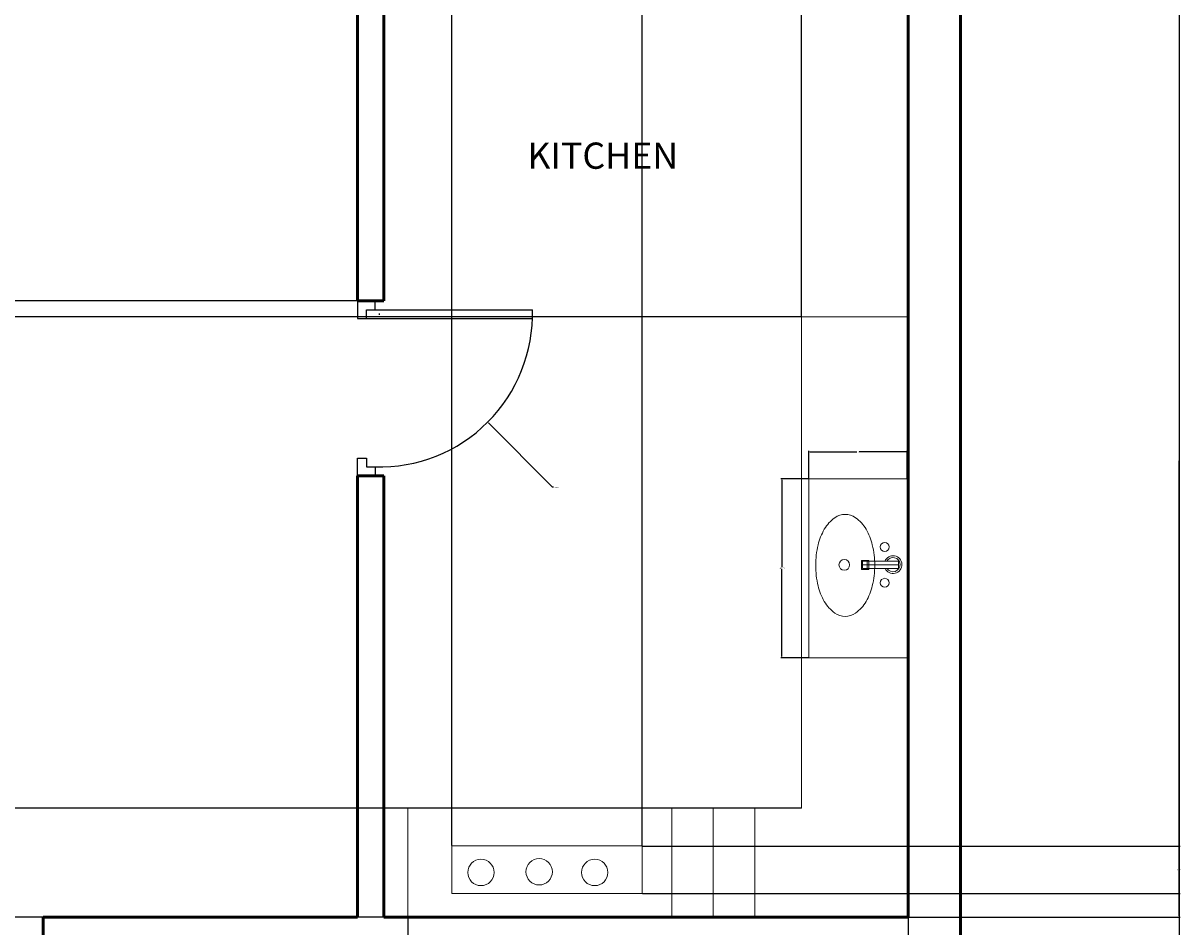
# Model space of a CAD drawing. Units: inches. Extents: x 1865 to 2541, y 1997 to 2759.
# Tile 10 of 11: x 2342 to 2541, y 2405 to 2560. Entities that reach past the tile are written whole.
import ezdxf

# ---------------------------------------------------------------- set-up
doc = ezdxf.new("R2010")
doc.units = ezdxf.units.IN
for name, color, linetype, lineweight in [('A-ANNO-DIMS', 2, 'Continuous', 18), ('A-AREA-IDEN', 4, 'Continuous', 18), ('A-EQPM', 8, 'Continuous', 18), ('A-FLOR-CASE', 8, 'Continuous', 20), ('A-FLOR-FIXT', 9, 'Continuous', 18), ('A-WALL', 7, 'Continuous', 50), ('DOOR', 1, 'Continuous', 25)]:
    doc.layers.add(name, color=color, linetype=linetype, lineweight=lineweight)
doc.styles.get("Standard").update_dxf_attribs({"font": 'arial.ttf'})
doc.dimstyles.get("Standard").update_dxf_attribs({"dimtxt": 0.18, "dimasz": 0.18, "dimexe": 0.18, "dimexo": 0.0625, "dimgap": 0.09, "dimtad": 0, "dimtih": 1, "dimtoh": 1, "dimdec": 4, "dimzin": 0, "dimdsep": 46, "dimtxsty": 'Standard', "dimcen": 0.09, "dimadec": 0, "dimazin": 0, "dimtfac": 1, "dimtdec": 4, "dimtofl": 0, "dimtmove": 0, "dimatfit": 3, "dimfxl": 1, "dimtolj": 1, "dimtzin": 0, "dimarcsym": 0})

# ---------------------------------------------------------------- blocks, each defined once
blk = doc.blocks.new('A$C50A015BB')
for p, q in [((0, 0.55), (1, 0.55)), ((0, 0.55), (0, 0)), ((1, 0.55), (1, 0)), ((0.4985, 0.5), (0.5385, 0.5)), ((0.4985, 0.5), (0.4985, 0.3)), ((0.5185, 0.5), (0.5185, 0.3)), ((0.5385, 0.5), (0.5385, 0.3)), ((0.4935, 0.335), (0.4935, 0.295)), ((0.4935, 0.335), (0.5435, 0.335)), ((0.4985, 0.325), (0.5385, 0.325)), ((0.5435, 0.335), (0.5435, 0.295)), ((0.4935, 0.295), (0.5435, 0.295)), ((0.4985, 0.3), (0.5385, 0.3)), ((0, 0), (1, 0)), ((0, 0), (1, 0))]:
    blk.add_line(p, q)
for centre, radius in [((0.4185, 0.424), 0.025), ((0.6185, 0.424), 0.025), ((0.5185, 0.1981), 0.0298)]:
    blk.add_circle(centre, radius)
for centre, radius, start, end in [((0.5201, 0.4703), 0.0497, 291.74253, 244.23308), ((0.5201, 0.4703), 0.0397, 297.63203, 237.02558), ((0.4772, 0.0383), 0.3252, 103.48533, 120.06859), ((0.5157, -0.1225), 0.4906, 90, 103.48533), ((0.5157, -0.1225), 0.4906, 76.51467, 90), ((0.5543, 0.0383), 0.3252, 59.93141, 76.51467), ((0.3299, 0.2031), 0.0991, 144.41781, 180), ((0.4185, 0.1397), 0.2081, 120.06859, 144.41781), ((0.613, 0.1397), 0.2081, 35.58219, 59.93141), ((0.7016, 0.2031), 0.0991, 0, 35.58219), ((0.3299, 0.2031), 0.0991, 180, 215.58219), ((0.7016, 0.2031), 0.0991, 324.41781, 0), ((0.4185, 0.2665), 0.2081, 215.58219, 239.93141), ((0.613, 0.2665), 0.2081, 300.06859, 324.41781), ((0.4772, 0.3679), 0.3252, 239.93141, 256.51467), ((0.5543, 0.3679), 0.3252, 283.48533, 300.06859), ((0.5157, 0.5288), 0.4906, 256.51467, 270), ((0.5157, 0.5288), 0.4906, 270, 283.48533)]:
    blk.add_arc(centre, radius, start, end)
blk = doc.blocks.new('DOOR-SWING-30IN')
for p, q in [((3, 30), (0, 30)), ((0, 30), (0, 27)), ((3, 28.5), (3, 30)), ((1.5, 27), (1.5, 28.5)), ((1.5, 28.5), (3, 28.5)), ((1.5, 28.5), (30, 28.5)), ((0, 27), (1.5, 27)), ((0, 27), (30, 27)), ((0, 0), (0, 3)), ((0, 3), (1.5, 3)), ((1.5, 3), (1.5, 1.5)), ((1.5, 1.5), (3, 1.5)), ((3, 1.5), (3, 0)), ((3, 0), (0, 0))]:
    blk.add_line(p, q)
blk.add_arc((3.75, 27.75), 26.26, 268.3634, 1.6366)
blk = doc.blocks.new('*D28')
at = {"layer": 'A-ANNO-DIMS', "color": 0, "lineweight": -2, "transparency": 16777216}
for p, q in [((2477.13, 2482.2), (2472.4, 2482.2)), ((2472.58, 2482.02), (2472.58, 2467.02)), ((2472.58, 2451.65), (2472.58, 2466.65)), ((2477.13, 2451.47), (2472.4, 2451.47))]:
    blk.add_line(p, q, dxfattribs=at)
at = {"layer": 'A-ANNO-DIMS', "color": 0, "transparency": 16777216}
for points in [[(2472.55, 2482.02), (2472.61, 2482.02), (2472.58, 2482.2)], [(2472.55, 2451.65), (2472.61, 2451.65), (2472.58, 2451.47)]]:
    blk.add_solid(points, dxfattribs=at)
at = {"layer": 'Defpoints', "color": 0, "transparency": 16777216}
for p in [(2472.58, 2482.2), (2477.19, 2482.2), (2477.19, 2451.47)]:
    blk.add_point(p, dxfattribs=at)
at = {"layer": 'A-ANNO-DIMS', "color": 0, "transparency": 16777216, "insert": (2472.58, 2466.83), "char_height": 0.18, "attachment_point": 5}
blk.add_mtext('\\A1;SINK 31', dxfattribs=at)
blk = doc.blocks.new('*D29')
at = {"layer": 'A-ANNO-DIMS', "color": 0, "lineweight": -2, "transparency": 16777216}
for p, q in [((2477.19, 2482.26), (2477.19, 2486.99)), ((2477.37, 2486.81), (2485.44, 2486.81)), ((2493.92, 2486.81), (2485.86, 2486.81)), ((2494.1, 2482.26), (2494.1, 2486.99))]:
    blk.add_line(p, q, dxfattribs=at)
at = {"layer": 'A-ANNO-DIMS', "color": 0, "transparency": 16777216}
for points in [[(2477.37, 2486.84), (2477.37, 2486.78), (2477.19, 2486.81)], [(2493.92, 2486.84), (2493.92, 2486.78), (2494.1, 2486.81)]]:
    blk.add_solid(points, dxfattribs=at)
at = {"layer": 'Defpoints', "color": 0, "transparency": 16777216}
for p in [(2494.1, 2486.81), (2477.19, 2482.2), (2494.1, 2482.2)]:
    blk.add_point(p, dxfattribs=at)
at = {"layer": 'A-ANNO-DIMS', "color": 0, "transparency": 16777216, "insert": (2485.65, 2486.81), "char_height": 0.18, "attachment_point": 5}
blk.add_mtext('\\A1;17', dxfattribs=at)
blk = doc.blocks.new('*D41')
at = {"layer": 'A-ANNO-DIMS', "color": 0, "lineweight": -2, "transparency": 16777216}
for p, q in [((2503.31, 2721.45), (2540.92, 2721.45)), ((2540.74, 2721.27), (2540.74, 2378.49)), ((2540.74, 2035.35), (2540.74, 2378.13)), ((2136.19, 2035.17), (2540.92, 2035.17))]:
    blk.add_line(p, q, dxfattribs=at)
at = {"layer": 'A-ANNO-DIMS', "color": 0, "transparency": 16777216}
for points in [[(2540.71, 2721.27), (2540.77, 2721.27), (2540.74, 2721.45)], [(2540.71, 2035.35), (2540.77, 2035.35), (2540.74, 2035.17)]]:
    blk.add_solid(points, dxfattribs=at)
at = {"layer": 'Defpoints', "color": 0, "transparency": 16777216}
for p in [(2503.24, 2721.45), (2136.13, 2035.17), (2540.74, 2035.17)]:
    blk.add_point(p, dxfattribs=at)
at = {"layer": 'A-ANNO-DIMS', "color": 0, "transparency": 16777216, "insert": (2540.74, 2378.31), "char_height": 0.18, "attachment_point": 5}
blk.add_mtext('\\A1;686.3', dxfattribs=at)
blk = doc.blocks.new('*D62')
at = {"layer": 'A-ANNO-DIMS', "color": 0, "lineweight": -2, "transparency": 16777216}
for p, q in [((2494.31, 2563.95), (2540.92, 2563.95)), ((2540.74, 2563.77), (2540.74, 2485.63)), ((2540.74, 2407.13), (2540.74, 2485.27)), ((2494.31, 2406.95), (2540.92, 2406.95))]:
    blk.add_line(p, q, dxfattribs=at)
at = {"layer": 'A-ANNO-DIMS', "color": 0, "transparency": 16777216}
for points in [[(2540.71, 2563.77), (2540.77, 2563.77), (2540.74, 2563.95)], [(2540.71, 2407.13), (2540.77, 2407.13), (2540.74, 2406.95)]]:
    blk.add_solid(points, dxfattribs=at)
at = {"layer": 'Defpoints', "color": 0, "transparency": 16777216}
for p in [(2494.24, 2563.95), (2540.74, 2563.95), (2494.24, 2406.95)]:
    blk.add_point(p, dxfattribs=at)
at = {"layer": 'A-ANNO-DIMS', "color": 0, "transparency": 16777216, "insert": (2540.74, 2485.45), "char_height": 0.18, "attachment_point": 5}
blk.add_mtext('\\A1;157', dxfattribs=at)
blk = doc.blocks.new('*D63')
at = {"layer": 'A-ANNO-DIMS', "color": 0, "lineweight": -2, "transparency": 16777216}
for p, q in [((2404.18, 2563.95), (1865.56, 2563.95)), ((1865.74, 2563.77), (1865.74, 2538.51)), ((1865.74, 2512.9), (1865.74, 2538.15)), ((2404.18, 2512.72), (1865.56, 2512.72))]:
    blk.add_line(p, q, dxfattribs=at)
at = {"layer": 'A-ANNO-DIMS', "color": 0, "transparency": 16777216}
for points in [[(1865.71, 2563.77), (1865.77, 2563.77), (1865.74, 2563.95)], [(1865.71, 2512.9), (1865.77, 2512.9), (1865.74, 2512.72)]]:
    blk.add_solid(points, dxfattribs=at)
at = {"layer": 'Defpoints', "color": 0, "transparency": 16777216}
for p in [(2404.24, 2563.95), (1865.74, 2512.72), (2404.24, 2512.72)]:
    blk.add_point(p, dxfattribs=at)
at = {"layer": 'A-ANNO-DIMS', "color": 0, "transparency": 16777216, "insert": (1865.74, 2538.33), "char_height": 0.18, "attachment_point": 5}
blk.add_mtext('\\A1;51.23', dxfattribs=at)
blk = doc.blocks.new('*D64')
at = {"layer": 'A-ANNO-DIMS', "color": 0, "lineweight": -2, "transparency": 16777216}
for p, q in [((2408.38, 2406.89), (2408.38, 1997.49)), ((2494.24, 2406.89), (2494.24, 1997.49)), ((2408.56, 1997.67), (2450.92, 1997.67)), ((2494.06, 1997.67), (2451.7, 1997.67))]:
    blk.add_line(p, q, dxfattribs=at)
at = {"layer": 'A-ANNO-DIMS', "color": 0, "transparency": 16777216}
for points in [[(2408.56, 1997.7), (2408.56, 1997.64), (2408.38, 1997.67)], [(2494.06, 1997.7), (2494.06, 1997.64), (2494.24, 1997.67)]]:
    blk.add_solid(points, dxfattribs=at)
at = {"layer": 'Defpoints', "color": 0, "transparency": 16777216}
for p in [(2408.38, 2406.95), (2494.24, 2406.95), (2494.24, 1997.67)]:
    blk.add_point(p, dxfattribs=at)
at = {"layer": 'A-ANNO-DIMS', "color": 0, "transparency": 16777216, "insert": (2451.31, 1997.67), "char_height": 0.18, "attachment_point": 5}
blk.add_mtext('\\A1;85.87', dxfattribs=at)
blk = doc.blocks.new('*D65')
at = {"layer": 'A-ANNO-DIMS', "color": 0, "lineweight": -2, "transparency": 16777216}
for p, q in [((2475.95, 2510.05), (2475.95, 2759.13)), ((2476.13, 2758.95), (2484.71, 2758.95)), ((2494.06, 2758.95), (2485.48, 2758.95)), ((2494.24, 2510.05), (2494.24, 2759.13))]:
    blk.add_line(p, q, dxfattribs=at)
at = {"layer": 'A-ANNO-DIMS', "color": 0, "transparency": 16777216}
for points in [[(2476.13, 2758.98), (2476.13, 2758.92), (2475.95, 2758.95)], [(2494.06, 2758.98), (2494.06, 2758.92), (2494.24, 2758.95)]]:
    blk.add_solid(points, dxfattribs=at)
at = {"layer": 'Defpoints', "color": 0, "transparency": 16777216}
for p in [(2494.24, 2758.95), (2475.95, 2509.99), (2494.24, 2509.99)]:
    blk.add_point(p, dxfattribs=at)
at = {"layer": 'A-ANNO-DIMS', "color": 0, "transparency": 16777216, "insert": (2485.1, 2758.95), "char_height": 0.18, "attachment_point": 5}
blk.add_mtext('\\A1;18.29', dxfattribs=at)
blk = doc.blocks.new('*D66')
at = {"layer": 'A-ANNO-DIMS', "color": 0, "lineweight": -2, "transparency": 16777216}
for p, q in [((2408.32, 2425.66), (1865.56, 2425.66)), ((1865.74, 2425.48), (1865.74, 2416.48)), ((1865.74, 2407.13), (1865.74, 2416.12)), ((2408.32, 2406.95), (1865.56, 2406.95))]:
    blk.add_line(p, q, dxfattribs=at)
at = {"layer": 'A-ANNO-DIMS', "color": 0, "transparency": 16777216}
for points in [[(1865.71, 2425.48), (1865.77, 2425.48), (1865.74, 2425.66)], [(1865.71, 2407.13), (1865.77, 2407.13), (1865.74, 2406.95)]]:
    blk.add_solid(points, dxfattribs=at)
at = {"layer": 'Defpoints', "color": 0, "transparency": 16777216}
for p in [(2408.38, 2425.66), (1865.74, 2406.95), (2408.38, 2406.95)]:
    blk.add_point(p, dxfattribs=at)
at = {"layer": 'A-ANNO-DIMS', "color": 0, "transparency": 16777216, "insert": (1865.74, 2416.3), "char_height": 0.18, "attachment_point": 5}
blk.add_mtext('\\A1;18.706', dxfattribs=at)
blk = doc.blocks.new('*D67')
at = {"layer": 'A-ANNO-DIMS', "color": 0, "lineweight": -2, "transparency": 16777216}
for p, q in [((2475.89, 2509.99), (1865.56, 2509.99)), ((1865.74, 2509.81), (1865.74, 2468)), ((1865.74, 2425.84), (1865.74, 2467.64)), ((2475.89, 2425.66), (1865.56, 2425.66))]:
    blk.add_line(p, q, dxfattribs=at)
at = {"layer": 'A-ANNO-DIMS', "color": 0, "transparency": 16777216}
for points in [[(1865.71, 2509.81), (1865.77, 2509.81), (1865.74, 2509.99)], [(1865.71, 2425.84), (1865.77, 2425.84), (1865.74, 2425.66)]]:
    blk.add_solid(points, dxfattribs=at)
at = {"layer": 'Defpoints', "color": 0, "transparency": 16777216}
for p in [(1865.74, 2509.99), (2475.95, 2509.99), (2475.95, 2425.66)]:
    blk.add_point(p, dxfattribs=at)
at = {"layer": 'A-ANNO-DIMS', "color": 0, "transparency": 16777216, "insert": (1865.74, 2467.82), "char_height": 0.18, "attachment_point": 5}
blk.add_mtext('\\A1;84.33', dxfattribs=at)
blk = doc.blocks.new('*D77')
at = {"layer": 'A-ANNO-DIMS', "color": 0, "lineweight": -2, "transparency": 16777216}
for p, q in [((2415.89, 2419.2), (2415.89, 2759.13)), ((2416.07, 2758.95), (2431.92, 2758.95)), ((2448.41, 2758.95), (2432.57, 2758.95)), ((2448.59, 2419.2), (2448.59, 2759.13))]:
    blk.add_line(p, q, dxfattribs=at)
at = {"layer": 'A-ANNO-DIMS', "color": 0, "transparency": 16777216}
for points in [[(2416.07, 2758.98), (2416.07, 2758.92), (2415.89, 2758.95)], [(2448.41, 2758.98), (2448.41, 2758.92), (2448.59, 2758.95)]]:
    blk.add_solid(points, dxfattribs=at)
at = {"layer": 'Defpoints', "color": 0, "transparency": 16777216}
for p in [(2448.59, 2758.95), (2415.89, 2419.14), (2448.59, 2419.14)]:
    blk.add_point(p, dxfattribs=at)
at = {"layer": 'A-ANNO-DIMS', "color": 0, "transparency": 16777216, "insert": (2432.24, 2758.95), "char_height": 0.18, "attachment_point": 5}
blk.add_mtext('\\A1;32.7', dxfattribs=at)
blk = doc.blocks.new('*D78')
at = {"layer": 'A-ANNO-DIMS', "color": 0, "lineweight": -2, "transparency": 16777216}
for p, q in [((2448.66, 2419.14), (2540.92, 2419.14)), ((2540.74, 2418.96), (2540.74, 2415.23)), ((2540.74, 2411.14), (2540.74, 2414.87)), ((2448.66, 2410.96), (2540.92, 2410.96))]:
    blk.add_line(p, q, dxfattribs=at)
at = {"layer": 'A-ANNO-DIMS', "color": 0, "transparency": 16777216}
for points in [[(2540.71, 2418.96), (2540.77, 2418.96), (2540.74, 2419.14)], [(2540.71, 2411.14), (2540.77, 2411.14), (2540.74, 2410.96)]]:
    blk.add_solid(points, dxfattribs=at)
at = {"layer": 'Defpoints', "color": 0, "transparency": 16777216}
for p in [(2448.59, 2419.14), (2448.59, 2410.96), (2540.74, 2410.96)]:
    blk.add_point(p, dxfattribs=at)
at = {"layer": 'A-ANNO-DIMS', "color": 0, "transparency": 16777216, "insert": (2540.74, 2415.05), "char_height": 0.18, "attachment_point": 5}
blk.add_mtext('\\A1;8.182', dxfattribs=at)
blk = doc.blocks.new('*D85')
at = {"layer": 'A-ANNO-DIMS', "color": 0, "lineweight": -2, "transparency": 16777216}
for p, q in [((2403.4, 2510.47), (2403.58, 2510.47)), ((2403.49, 2510.38), (2403.49, 2510.56)), ((2433.2, 2480.76), (2422.19, 2491.77)), ((2433.38, 2480.76), (2433.2, 2480.76))]:
    blk.add_line(p, q, dxfattribs=at)
at = {"layer": 'A-ANNO-DIMS', "color": 0, "transparency": 16777216}
blk.add_solid([(2422.21, 2491.79), (2422.17, 2491.75), (2422.06, 2491.9)], dxfattribs=at)
at = {"layer": 'Defpoints', "color": 0, "transparency": 16777216}
for p in [(2403.49, 2510.47), (2422.06, 2491.9)]:
    blk.add_point(p, dxfattribs=at)
at = {"layer": 'A-ANNO-DIMS', "color": 0, "transparency": 16777216, "insert": (2433.86, 2480.76), "char_height": 0.18, "attachment_point": 5}
blk.add_mtext('\\A1;R26.26', dxfattribs=at)

msp = doc.modelspace()

# ---------------------------------------------------------------- linework, layer by layer
at = {"layer": 'A-EQPM'}
msp.add_lwpolyline([(2415.893, 2410.9604), (2415.893, 2419.142), (2448.5933, 2419.142), (2448.5933, 2410.9604)], close=True, dxfattribs=at)
for centre in [(2420.9127, 2414.598), (2430.9038, 2414.713), (2440.4356, 2414.598)]:
    msp.add_circle(centre, 2.2624, dxfattribs=at)
at = {"layer": 'A-FLOR-CASE'}
for p, q in [((2494.243, 2509.9875), (2475.9518, 2509.9875)), ((2475.9518, 2509.9875), (2475.9518, 2425.6552)), ((2494.243, 2406.9494), (2494.243, 2509.9875)), ((2408.3779, 2406.9494), (2408.3779, 2425.6552)), ((2408.3779, 2425.6552), (2475.9518, 2425.6552)), ((2460.7921, 2406.9494), (2460.7921, 2425.6552)), ((2494.243, 2406.9494), (2408.3779, 2406.9494))]:
    msp.add_line(p, q, dxfattribs=at)
msp.add_lwpolyline([(2453.6572, 2406.9494), (2453.6572, 2425.6552), (2467.9269, 2425.6552), (2467.9269, 2406.9494)], close=True, dxfattribs=at)
at = {"layer": 'A-WALL'}
for p, q in [((2503.243, 2061.4494), (2503.243, 2721.4494)), ((2399.743, 2512.7166), (2399.743, 2563.9494)), ((2404.243, 2512.7166), (2404.243, 2563.9494)), ((2494.243, 2406.9494), (2494.243, 2563.9494)), ((2399.743, 2512.7166), (2404.243, 2512.7166)), ((2399.743, 2406.9494), (2399.743, 2482.7166)), ((2399.743, 2482.7166), (2404.243, 2482.7166)), ((2404.243, 2406.9494), (2404.243, 2482.7166)), ((2399.743, 2406.9494), (2345.743, 2406.9494)), ((2345.743, 2402.4494), (2345.743, 2406.9494)), ((2494.243, 2406.9494), (2404.243, 2406.9494))]:
    msp.add_line(p, q, dxfattribs=at)

# ---------------------------------------------------------------- block references
at = {"layer": 'A-FLOR-FIXT', "xscale": -30.73195797824049, "yscale": 30.73195797824049, "zscale": 30.73195797824049, "rotation": 270}
msp.add_blockref('A$C50A015BB', (2477.1943, 2451.467), dxfattribs=at)
at = {"layer": 'DOOR'}
msp.add_blockref('DOOR-SWING-30IN', (2399.743, 2482.717), dxfattribs=at)

# ---------------------------------------------------------------- texts
at = {"layer": 'A-AREA-IDEN', "insert": (2428.8768, 2539.9076), "char_height": 4.5, "attachment_point": 1}
msp.add_mtext_dynamic_manual_height_columns('KITCHEN', width=66.075761, gutter_width=12.5, heights=[0], dxfattribs=at)

# ---------------------------------------------------------------- dimensions: what is measured, and where the dimension line sits
at = {"layer": 'A-ANNO-DIMS'}
for base, p1, p2, override, picture, middle in [((2448.5933, 2758.9494), (2415.893, 2419.142), (2448.5933, 2419.142), {"dimdec": 1, "dimlfac": 1, "dimrnd": 0, "dimzin": 0, "dimdsep": 46, "dimlunit": 2}, '*D77', (2432.2431, 2758.9494)), ((2494.243, 2758.9494), (2475.9518, 2509.9875), (2494.243, 2509.9875), {"dimdec": 2, "dimlfac": 1, "dimrnd": 0, "dimzin": 0, "dimdsep": 46, "dimlunit": 2}, '*D65', (2485.0974, 2758.9494)), ((2494.0969, 2486.8088), (2477.1943, 2482.199), (2494.0969, 2482.199), {"dimdec": 0, "dimlfac": 1, "dimrnd": 0, "dimzin": 0, "dimdsep": 46, "dimlunit": 2}, '*D29', (2485.6456, 2486.8088)), ((2494.243, 1997.6708), (2408.3779, 2406.9494), (2494.243, 2406.9494), {"dimdec": 2, "dimlfac": 1, "dimrnd": 0, "dimzin": 0, "dimdsep": 46, "dimlunit": 2}, '*D64', (2451.3105, 1997.6708))]:
    dim = msp.add_linear_dim(base=base, p1=p1, p2=p2, dimstyle='Standard', override=override, dxfattribs=at)
    dim.commit()
    dim.dimension.update_dxf_attribs({"geometry": picture, "text_midpoint": middle})
for base, p1, p2, override, picture, middle in [((2540.743, 2035.1708), (2503.243, 2721.4494), (2136.13, 2035.1708), {"dimdec": 1, "dimlfac": 1, "dimrnd": 0, "dimzin": 0, "dimdsep": 46, "dimlunit": 2}, '*D41', (2540.743, 2378.3101)), ((1865.743, 2512.7166), (2404.243, 2563.9494), (2404.243, 2512.7166), {"dimdec": 2, "dimlfac": 1, "dimrnd": 0, "dimzin": 0, "dimdsep": 46, "dimlunit": 2}, '*D63', (1865.743, 2538.333)), ((2540.743, 2563.9494), (2494.243, 2406.9494), (2494.243, 2563.9494), {"dimdec": 0, "dimlfac": 1, "dimrnd": 0, "dimzin": 0, "dimdsep": 46, "dimlunit": 2}, '*D62', (2540.743, 2485.4494)), ((1865.743, 2509.9875), (2475.9518, 2425.6552), (2475.9518, 2509.9875), {"dimdec": 2, "dimlfac": 1, "dimrnd": 0, "dimzin": 0, "dimdsep": 46, "dimlunit": 2}, '*D67', (1865.743, 2467.8214)), ((1865.743, 2406.9494), (2408.3779, 2425.6552), (2408.3779, 2406.9494), {"dimdec": 3, "dimlfac": 1, "dimrnd": 0, "dimzin": 0, "dimdsep": 46, "dimlunit": 2}, '*D66', (1865.743, 2416.3023)), ((2540.743, 2410.9604), (2448.5933, 2419.142), (2448.5933, 2410.9604), {"dimdec": 3, "dimlfac": 1, "dimrnd": 0, "dimzin": 0, "dimdsep": 46, "dimlunit": 2}, '*D78', (2540.743, 2415.0512))]:
    dim = msp.add_linear_dim(base=base, p1=p1, p2=p2, angle=90, dimstyle='Standard', override=override, dxfattribs=at)
    dim.commit()
    dim.dimension.update_dxf_attribs({"geometry": picture, "text_midpoint": middle})
dim = msp.add_radius_dim(center=(2403.493, 2510.4666), mpoint=(2422.0618, 2491.8972), dimstyle='Standard', override={"dimdec": 2, "dimlfac": 1, "dimrnd": 0, "dimzin": 0, "dimdsep": 46, "dimlunit": 2}, dxfattribs=at)
dim.commit()
dim.dimension.update_dxf_attribs({"geometry": '*D85', "text_midpoint": (2433.8629, 2480.7555), "dimtype": 164})
dim = msp.add_linear_dim(base=(2472.5846, 2482.199), p1=(2477.1943, 2451.467), p2=(2477.1943, 2482.199), angle=90, text='SINK <>', dimstyle='Standard', override={"dimdec": 0, "dimlfac": 1, "dimrnd": 0, "dimzin": 0, "dimdsep": 46, "dimlunit": 2}, dxfattribs=at)
dim.commit()
dim.dimension.update_dxf_attribs({"geometry": '*D28', "text_midpoint": (2472.5846, 2466.833)})

doc.saveas('drawing.dxf')
